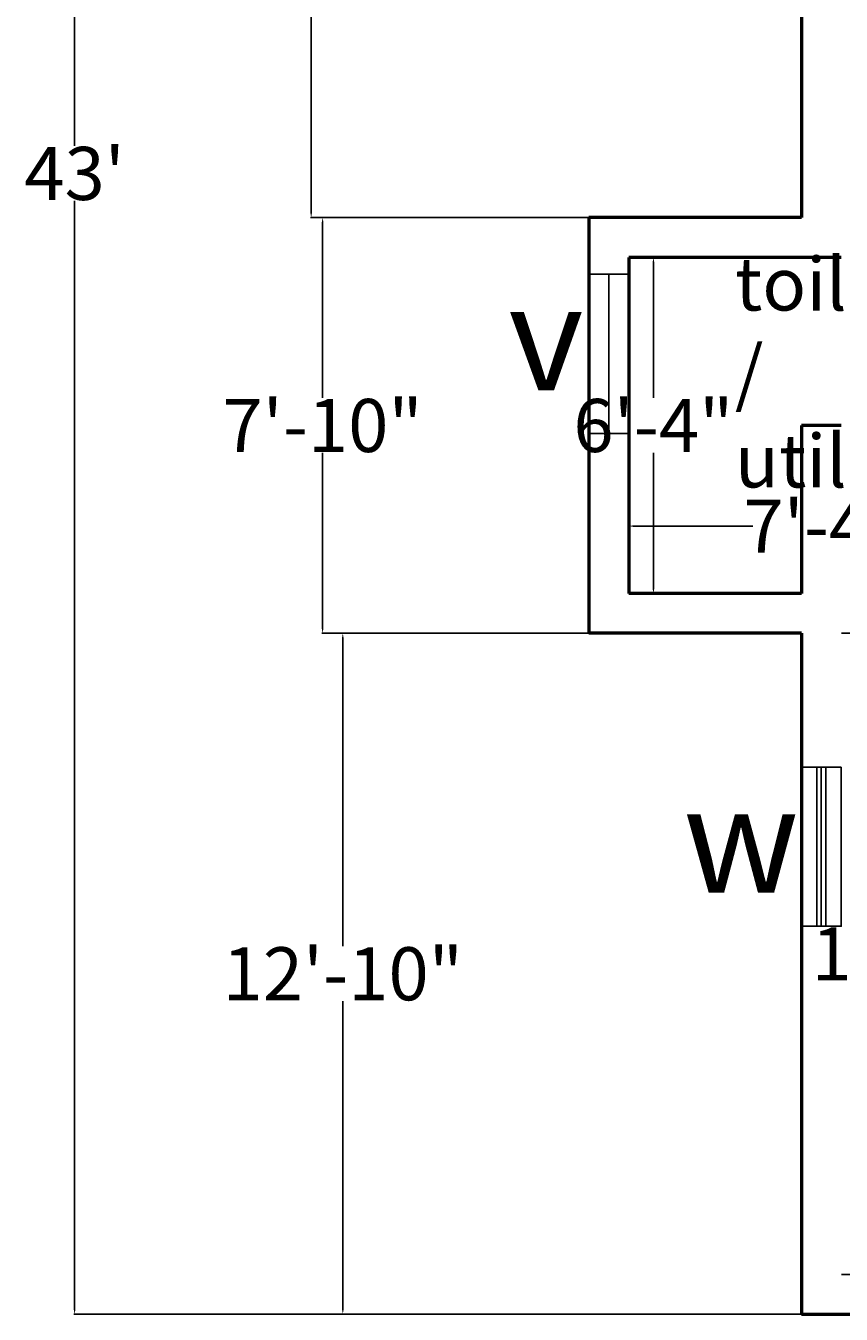
# Model space of a CAD drawing. Units: inches. Extents: x 409 to 7572, y 7 to 725.
# Tile 21 of 38: x 4151 to 4335, y 157 to 448. Entities that reach past the tile are written whole.
import ezdxf

# ---------------------------------------------------------------- set-up
doc = ezdxf.new("R2010")
doc.units = ezdxf.units.IN
doc.header["$MEASUREMENT"] = 0
for name, color, linetype, lineweight in [('A-ANNO-DIMS', 2, 'Continuous', 18), ('A-ANNO-SYMB', 3, 'Continuous', 25), ('A-AREA-IDEN', 7, 'Continuous', 25), ('A-GLAZ', 4, 'Continuous', 25), ('A-WALL', 7, 'Continuous', 50)]:
    doc.layers.add(name, color=color, linetype=linetype, lineweight=lineweight)
doc.styles.get("Standard").update_dxf_attribs({"font": 'arial.ttf'})
doc.dimstyles.get("Standard").update_dxf_attribs({"dimtxt": 2, "dimasz": 1, "dimexe": 0.18, "dimexo": 0.0625, "dimgap": 0.09, "dimtad": 0, "dimtih": 1, "dimtoh": 1, "dimdec": 0, "dimzin": 0, "dimdsep": 46, "dimlunit": 3, "dimtxsty": 'Standard', "dimcen": 0.09, "dimadec": 0, "dimazin": 0, "dimtfac": 1, "dimtdec": 0, "dimtofl": 0, "dimtmove": 0, "dimatfit": 3, "dimfxl": 1, "dimtolj": 1, "dimtzin": 0, "dimarcsym": 0})

# ---------------------------------------------------------------- blocks, each defined once
blk = doc.blocks.new('*D98')
at = {"layer": 'A-ANNO-DIMS', "color": 0, "lineweight": -2, "transparency": 16777216}
for p, q in [((4335, 310.53), (4351.04, 310.53)), ((4350.86, 309.53), (4350.86, 244.15)), ((4350.86, 166.53), (4350.86, 231.92)), ((4335, 165.53), (4351.04, 165.53))]:
    blk.add_line(p, q, dxfattribs=at)
at = {"layer": 'A-ANNO-DIMS', "color": 0, "transparency": 16777216}
for points in [[(4350.7, 309.53), (4351.03, 309.53), (4350.86, 310.53)], [(4350.7, 166.53), (4351.03, 166.53), (4350.86, 165.53)]]:
    blk.add_solid(points, dxfattribs=at)
at = {"layer": 'DEFPOINTS', "color": 0, "transparency": 16777216}
for p in [(4334.94, 310.53), (4334.94, 165.53), (4350.86, 165.53)]:
    blk.add_point(p, dxfattribs=at)
at = {"layer": 'A-ANNO-DIMS', "color": 0, "transparency": 16777216, "insert": (4350.86, 238.03), "char_height": 2, "attachment_point": 5}
blk.add_mtext('\\A1;{\\H6x;12\'-1"}', dxfattribs=at)
blk = doc.blocks.new('*D115')
at = {"layer": 'A-ANNO-DIMS', "color": 0, "lineweight": -2, "transparency": 16777216}
for p, q in [((4296.14, 395.53), (4292.32, 395.53)), ((4292.5, 394.53), (4292.5, 363.75)), ((4292.5, 320.53), (4292.5, 351.31)), ((4296.14, 319.53), (4292.32, 319.53))]:
    blk.add_line(p, q, dxfattribs=at)
at = {"layer": 'A-ANNO-DIMS', "color": 0, "transparency": 16777216}
for points in [[(4292.34, 394.53), (4292.67, 394.53), (4292.5, 395.53)], [(4292.34, 320.53), (4292.67, 320.53), (4292.5, 319.53)]]:
    blk.add_solid(points, dxfattribs=at)
at = {"layer": 'DEFPOINTS', "color": 0, "transparency": 16777216}
for p in [(4296.21, 395.53), (4292.5, 319.53), (4296.21, 319.53)]:
    blk.add_point(p, dxfattribs=at)
at = {"layer": 'A-ANNO-DIMS', "color": 0, "transparency": 16777216, "insert": (4292.5, 357.53), "char_height": 2, "attachment_point": 5}
blk.add_mtext('\\A1;{\\H6x;6\'-4"}', dxfattribs=at)
blk = doc.blocks.new('*D117')
at = {"layer": 'A-ANNO-DIMS', "color": 0, "lineweight": -2, "transparency": 16777216}
for p, q in [((4286.94, 346.33), (4286.94, 334.6)), ((4374.94, 346.33), (4374.94, 334.6)), ((4287.94, 334.78), (4314.95, 334.78)), ((4373.94, 334.78), (4346.93, 334.78))]:
    blk.add_line(p, q, dxfattribs=at)
at = {"layer": 'A-ANNO-DIMS', "color": 0, "transparency": 16777216}
for points in [[(4287.94, 334.95), (4287.94, 334.61), (4286.94, 334.78)], [(4373.94, 334.95), (4373.94, 334.61), (4374.94, 334.78)]]:
    blk.add_solid(points, dxfattribs=at)
at = {"layer": 'DEFPOINTS', "color": 0, "transparency": 16777216}
for p in [(4286.94, 346.39), (4374.94, 346.39), (4374.94, 334.78)]:
    blk.add_point(p, dxfattribs=at)
at = {"layer": 'A-ANNO-DIMS', "color": 0, "transparency": 16777216, "insert": (4330.94, 334.78), "char_height": 2, "attachment_point": 5}
blk.add_mtext('\\A1;{\\H6x;7\'-4"}', dxfattribs=at)
blk = doc.blocks.new('*D104')
at = {"layer": 'A-ANNO-DIMS', "color": 0, "lineweight": -2, "transparency": 16777216}
for p, q in [((4325.88, 672.53), (4214.98, 672.53)), ((4215.16, 671.53), (4215.16, 544.65)), ((4215.16, 405.53), (4215.16, 532.42)), ((4325.88, 404.53), (4214.98, 404.53))]:
    blk.add_line(p, q, dxfattribs=at)
at = {"layer": 'A-ANNO-DIMS', "color": 0, "transparency": 16777216}
for points in [[(4214.99, 671.53), (4215.33, 671.53), (4215.16, 672.53)], [(4214.99, 405.53), (4215.33, 405.53), (4215.16, 404.53)]]:
    blk.add_solid(points, dxfattribs=at)
at = {"layer": 'DEFPOINTS', "color": 0, "transparency": 16777216}
for p in [(4325.94, 672.53), (4215.16, 404.53), (4325.94, 404.53)]:
    blk.add_point(p, dxfattribs=at)
at = {"layer": 'A-ANNO-DIMS', "color": 0, "transparency": 16777216, "insert": (4215.16, 538.53), "char_height": 2, "attachment_point": 5}
blk.add_mtext('\\A1;{\\H6x;22\'-4"}', dxfattribs=at)
blk = doc.blocks.new('*D105')
at = {"layer": 'A-ANNO-DIMS', "color": 0, "lineweight": -2, "transparency": 16777216}
for p, q in [((4277.88, 404.53), (4217.57, 404.53)), ((4217.75, 403.53), (4217.75, 363.75)), ((4217.75, 311.53), (4217.75, 351.31)), ((4277.88, 310.53), (4217.57, 310.53))]:
    blk.add_line(p, q, dxfattribs=at)
at = {"layer": 'A-ANNO-DIMS', "color": 0, "transparency": 16777216}
for points in [[(4217.58, 403.53), (4217.92, 403.53), (4217.75, 404.53)], [(4217.58, 311.53), (4217.92, 311.53), (4217.75, 310.53)]]:
    blk.add_solid(points, dxfattribs=at)
at = {"layer": 'DEFPOINTS', "color": 0, "transparency": 16777216}
for p in [(4277.94, 404.53), (4217.75, 310.53), (4277.94, 310.53)]:
    blk.add_point(p, dxfattribs=at)
at = {"layer": 'A-ANNO-DIMS', "color": 0, "transparency": 16777216, "insert": (4217.75, 357.53), "char_height": 2, "attachment_point": 5}
blk.add_mtext('\\A1;{\\H6x;7\'-10"}', dxfattribs=at)
blk = doc.blocks.new('*D106')
at = {"layer": 'A-ANNO-DIMS', "color": 0, "lineweight": -2, "transparency": 16777216}
for p, q in [((4325.88, 310.53), (4222.13, 310.53)), ((4222.31, 309.53), (4222.31, 239.75)), ((4222.31, 157.53), (4222.31, 227.31)), ((4325.88, 156.53), (4222.13, 156.53))]:
    blk.add_line(p, q, dxfattribs=at)
at = {"layer": 'A-ANNO-DIMS', "color": 0, "transparency": 16777216}
for points in [[(4222.14, 309.53), (4222.48, 309.53), (4222.31, 310.53)], [(4222.14, 157.53), (4222.48, 157.53), (4222.31, 156.53)]]:
    blk.add_solid(points, dxfattribs=at)
at = {"layer": 'DEFPOINTS', "color": 0, "transparency": 16777216}
for p in [(4325.94, 310.53), (4222.31, 156.53), (4325.94, 156.53)]:
    blk.add_point(p, dxfattribs=at)
at = {"layer": 'A-ANNO-DIMS', "color": 0, "transparency": 16777216, "insert": (4222.31, 233.53), "char_height": 2, "attachment_point": 5}
blk.add_mtext('\\A1;{\\H6x;12\'-10"}', dxfattribs=at)
blk = doc.blocks.new('*D93')
at = {"layer": 'A-ANNO-DIMS', "color": 0, "lineweight": -2, "transparency": 16777216}
for p, q in [((4325.88, 672.53), (4161.52, 672.53)), ((4161.7, 671.53), (4161.7, 420.75)), ((4161.7, 157.53), (4161.7, 408.31)), ((4325.88, 156.53), (4161.52, 156.53))]:
    blk.add_line(p, q, dxfattribs=at)
at = {"layer": 'A-ANNO-DIMS', "color": 0, "transparency": 16777216}
for points in [[(4161.54, 671.53), (4161.87, 671.53), (4161.7, 672.53)], [(4161.54, 157.53), (4161.87, 157.53), (4161.7, 156.53)]]:
    blk.add_solid(points, dxfattribs=at)
at = {"layer": 'DEFPOINTS', "color": 0, "transparency": 16777216}
for p in [(4325.94, 672.53), (4161.7, 156.53), (4325.94, 156.53)]:
    blk.add_point(p, dxfattribs=at)
at = {"layer": 'A-ANNO-DIMS', "color": 0, "transparency": 16777216, "insert": (4161.7, 414.53), "char_height": 2, "attachment_point": 5}
blk.add_mtext("\\A1;{\\H6x;43'}", dxfattribs=at)
blk = doc.blocks.new('WIN-36')
for p, q in [((1699.82, 514.65), (1699.82, 478.65)), ((1700.82, 514.65), (1700.82, 478.65)), ((1701.82, 514.65), (1701.82, 478.65))]:
    blk.add_line(p, q)
blk.add_lwpolyline([(1705.32, 514.65), (1705.32, 478.65), (1696.32, 478.65), (1696.32, 514.65)], close=True)
blk = doc.blocks.new('VENT-36')
blk.add_line((5633.28, 355.73), (5633.28, 391.73))
blk.add_lwpolyline([(5628.78, 355.73), (5628.78, 391.73), (5637.78, 391.73), (5637.78, 355.73)], close=True)

msp = doc.modelspace()

# ---------------------------------------------------------------- linework, layer by layer
at = {"layer": 'A-WALL'}
for p, q in [((4325.94, 672.53), (4325.94, 404.53)), ((4325.94, 404.53), (4277.94, 404.53)), ((4277.94, 404.53), (4277.94, 310.53)), ((4334.94, 395.53), (4286.94, 395.53)), ((4286.94, 395.53), (4286.94, 319.53)), ((4325.94, 357.53), (4325.94, 319.53)), ((4334.94, 357.53), (4325.94, 357.53)), ((4325.94, 319.53), (4286.94, 319.53)), ((4325.94, 310.53), (4277.94, 310.53)), ((4325.94, 310.53), (4325.94, 156.53)), ((4325.94, 156.53), (4699.94, 156.53))]:
    msp.add_line(p, q, dxfattribs=at)

# ---------------------------------------------------------------- block references
at = {"layer": 'A-GLAZ'}
for name, p in [('VENT-36', (-1350.84, 0)), ('WIN-36', (2629.62, -234.38))]:
    msp.add_blockref(name, p, dxfattribs=at)

# ---------------------------------------------------------------- texts
at = {"layer": 'A-ANNO-SYMB', "char_height": 24, "attachment_point": 1}
for s, insert in [('v', (4259.68, 389.45)), ('w', (4299.18, 275.84))]:
    msp.add_mtext_dynamic_manual_height_columns(s, width=18.2582, gutter_width=1, heights=[0], dxfattribs=dict(at, insert=insert))
at = {"layer": 'A-AREA-IDEN', "insert": (4310.94, 395.53), "char_height": 12, "attachment_point": 1}
msp.add_mtext_dynamic_manual_height_columns('toilet / utility', width=49.2946, gutter_width=1, heights=[0], dxfattribs=at)

# ---------------------------------------------------------------- dimensions: what is measured, and where the dimension line sits
at = {"layer": 'A-ANNO-DIMS'}
for base, p1, p2, picture, middle in [((4161.7, 156.53), (4325.94, 672.53), (4325.94, 156.53), '*D93', (4161.7, 414.53)), ((4215.16, 404.53), (4325.94, 672.53), (4325.94, 404.53), '*D104', (4215.16, 538.53)), ((4217.75, 310.53), (4277.94, 404.53), (4277.94, 310.53), '*D105', (4217.75, 357.53)), ((4292.5, 319.53), (4296.21, 395.53), (4296.21, 319.53), '*D115', (4292.5, 357.53)), ((4222.31, 156.53), (4325.94, 310.53), (4325.94, 156.53), '*D106', (4222.31, 233.53)), ((4350.86, 165.53), (4334.94, 310.53), (4334.94, 165.53), '*D98', (4350.86, 238.03))]:
    dim = msp.add_linear_dim(base=base, p1=p1, p2=p2, angle=90, text='{\\H6x;<>}', dimstyle='Standard', override={"dimclrd": 0, "dimclre": 0, "dimclrt": 0}, dxfattribs=at)
    dim.commit()
    dim.dimension.update_dxf_attribs({"geometry": picture, "text_midpoint": middle})
dim = msp.add_linear_dim(base=(4374.94, 334.78), p1=(4286.94, 346.39), p2=(4374.94, 346.39), text='{\\H6x;<>}', dimstyle='Standard', override={"dimclrd": 0, "dimclre": 0, "dimclrt": 0}, dxfattribs=at)
dim.commit()
dim.dimension.update_dxf_attribs({"geometry": '*D117', "text_midpoint": (4330.94, 334.78)})

doc.saveas('drawing.dxf')
